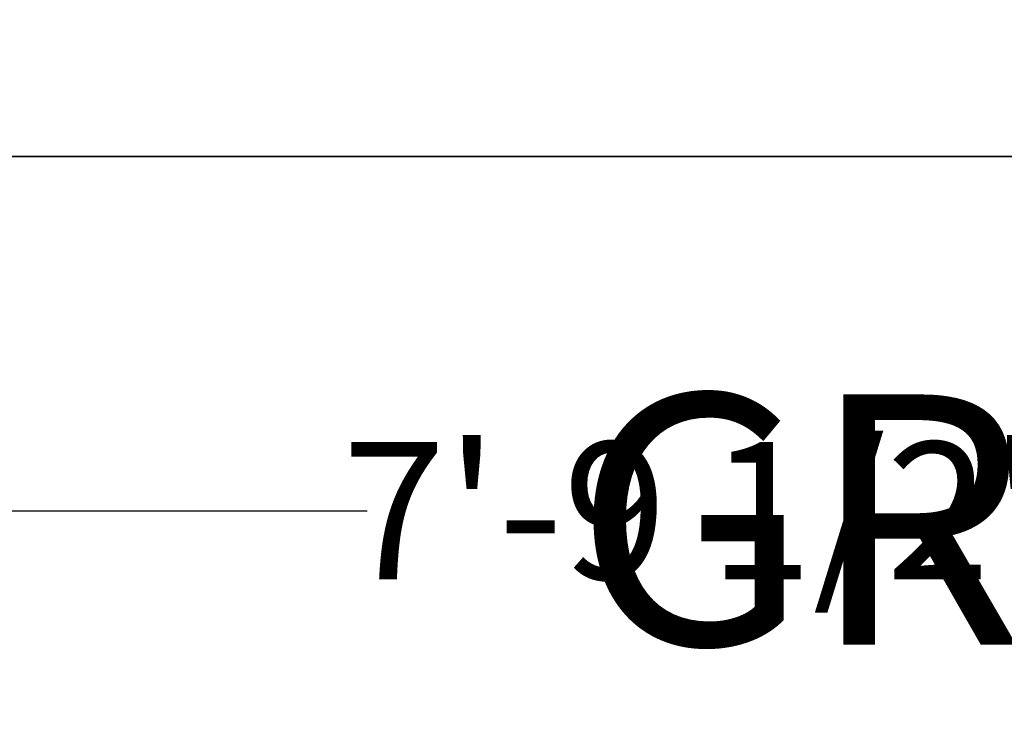
# Model space of a CAD drawing. Units: inches. Extents: x -4737294 to -4736756, y 1716389 to 1717040.
# Tile 2 of 25: x -4737190 to -4737133, y 1716424 to 1716465. Entities that reach past the tile are written whole.
import ezdxf

# ---------------------------------------------------------------- set-up
doc = ezdxf.new("R2010")
doc.units = ezdxf.units.IN
doc.header["$MEASUREMENT"] = 0
for name, color, linetype, lineweight in [('A-ANNO-DIMS', 2, 'Continuous', 18), ('A-ANNO-TEXT', 250, 'Continuous', 30), ('walls', 252, 'Continuous', 35)]:
    doc.layers.add(name, color=color, linetype=linetype, lineweight=lineweight)
doc.styles.get("Standard").update_dxf_attribs({"font": 'arial.ttf'})
doc.dimstyles.get("Standard").update_dxf_attribs({"dimtxt": 8, "dimasz": 0.18, "dimexe": 0.18, "dimexo": 0.0625, "dimgap": 0.09, "dimtad": 0, "dimtih": 1, "dimtoh": 1, "dimzin": 0, "dimdsep": 46, "dimlunit": 3, "dimtxsty": 'Standard', "dimcen": 0.09, "dimadec": 0, "dimazin": 0, "dimtfac": 1, "dimtofl": 0, "dimtmove": 0, "dimatfit": 3, "dimfxl": 1, "dimtolj": 1, "dimtzin": 0, "dimarcsym": 0})

# ---------------------------------------------------------------- blocks, each defined once
blk = doc.blocks.new('*D60')
at = {"layer": 'A-ANNO-DIMS', "color": 0, "lineweight": -2, "transparency": 16777216}
for p, q in [((-4737196.476, 1716464.781), (-4737196.476, 1716436.041)), ((-4737102.951, 1716464.781), (-4737102.951, 1716436.041)), ((-4737196.296, 1716436.221), (-4737169.725, 1716436.221)), ((-4737103.131, 1716436.221), (-4737129.703, 1716436.221))]:
    blk.add_line(p, q, dxfattribs=at)
at = {"layer": 'A-ANNO-DIMS', "color": 0, "transparency": 16777216}
for points in [[(-4737196.296, 1716436.251), (-4737196.296, 1716436.191), (-4737196.476, 1716436.221)], [(-4737103.131, 1716436.251), (-4737103.131, 1716436.191), (-4737102.951, 1716436.221)]]:
    blk.add_solid(points, dxfattribs=at)
at = {"layer": 'Defpoints', "color": 0, "transparency": 16777216}
for p in [(-4737196.476, 1716464.844), (-4737102.951, 1716464.844), (-4737102.951, 1716436.221)]:
    blk.add_point(p, dxfattribs=at)
at = {"layer": 'A-ANNO-DIMS', "color": 0, "transparency": 16777216, "insert": (-4737149.714, 1716436.221), "char_height": 8, "attachment_point": 5}
blk.add_mtext('\\A1;7\'-9 1/2"', dxfattribs=at)

msp = doc.modelspace()

# ---------------------------------------------------------------- linework, layer by layer
at = {"layer": 'walls'}
msp.add_line((-4737215.144, 1716456.869), (-4737062.144, 1716456.869), dxfattribs=at)

# ---------------------------------------------------------------- texts
at = {"layer": 'A-ANNO-TEXT'}
msp.add_text('GROUND FLOOR PLAN', height=14.58777, dxfattribs=at).set_placement((-4737157.681, 1716428.409))

# ---------------------------------------------------------------- dimensions: what is measured, and where the dimension line sits
at = {"layer": 'A-ANNO-DIMS'}
dim = msp.add_linear_dim(base=(-4737102.951, 1716436.221), p1=(-4737196.476, 1716464.844), p2=(-4737102.951, 1716464.844), dimstyle='Standard', override={"dimdec": 1, "dimlfac": 1, "dimrnd": 0, "dimzin": 1, "dimdsep": 46, "dimlunit": 4, "dimfrac": 2}, dxfattribs=at)
dim.commit()
dim.dimension.update_dxf_attribs({"geometry": '*D60', "text_midpoint": (-4737149.714, 1716436.221)})

doc.saveas('drawing.dxf')
